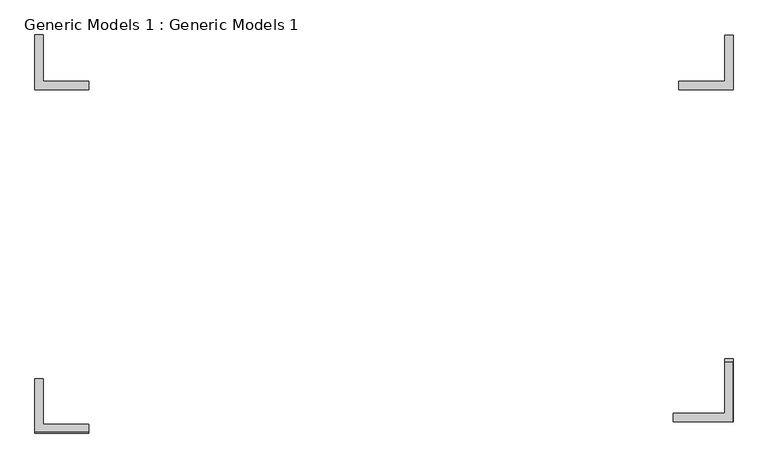
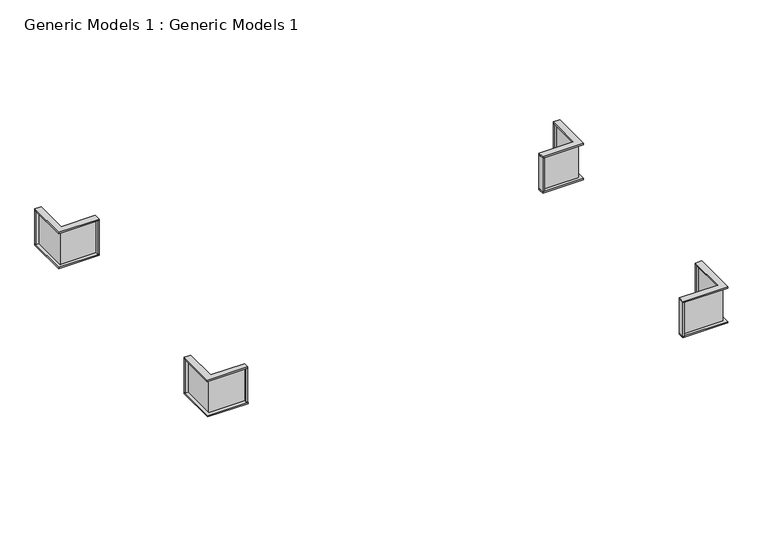
"""IFC4 building model written with IfcOpenShell, lengths in millimetres: proxy geometry, Generic Models 1 : Generic Models 1."""

from ifc_helpers import new_model, si_unit, frame, origin, place, context, project, spatial, polyline, outline, extrude, source, transform, mapped, element, save


def generic_models_1_generic_models_1_b24af07e(model_context):
    return source(origin(), model_context, "Body", "SweptSolid", [
        extrude(outline(polyline([(-6988.9378503, -5640.2673024), (-6988.9378503, -4368.6481466), (-6963.5378503, -4368.6481466), (-6963.5378503, -5614.8673024), (-5709.5498785, -5614.8673024), (-5709.5498785, -5640.2673024), (-6988.9378503, -5640.2673024)])), frame((0.0, 0.0, 4114.8), z_axis=(0.0, 0.0, 1.0), x_axis=(1.0, 0.0, 0.0)), (0.0, 0.0, 1.0), 1320.8),
        extrude(outline(polyline([(-6988.9378503, 3565.6135417), (-6988.9378503, 4868.3012615), (-6963.5378503, 4868.3012615), (-6963.5378503, 3591.0135417), (-5711.2501867, 3591.0135417), (-5711.2501867, 3565.6135417), (-6988.9378503, 3565.6135417)])), frame((0.0, 0.0, 4114.8), z_axis=(0.0, 0.0, 1.0), x_axis=(1.0, 0.0, 0.0)), (0.0, 0.0, 1.0), 1320.8),
        extrude(outline(polyline([(-7103.2378503, 4919.1012615), (-6874.6378503, 4919.1012615), (-6874.6378503, 4868.3012615), (-7103.2378503, 4868.3012615), (-7103.2378503, 4919.1012615)])), frame((0.0, 0.0, 4165.6), z_axis=(0.0, 0.0, 1.0), x_axis=(1.0, 0.0, 0.0)), (0.0, 0.0, 1.0), 1270.0),
        extrude(outline(polyline([(-5660.4501867, 3679.9135417), (-5660.4501867, 3451.3135417), (-5711.2501867, 3451.3135417), (-5711.2501867, 3679.9135417), (-5660.4501867, 3679.9135417)])), frame((0.0, 0.0, 4165.6), z_axis=(0.0, 0.0, 1.0), x_axis=(1.0, 0.0, 0.0)), (0.0, 0.0, 1.0), 1270.0),
        extrude(outline(polyline([(-7103.2378503, 3451.3135417), (-7103.2378503, 4919.1012615), (-6874.6378503, 4919.1012615), (-6874.6378503, 3679.9135417), (-5660.4501867, 3679.9135417), (-5660.4501867, 3451.3135417), (-7103.2378503, 3451.3135417)])), frame((0.0, 0.0, 5435.6), z_axis=(0.0, 0.0, 1.0), x_axis=(1.0, 0.0, 0.0)), (0.0, 0.0, 1.0), 50.8),
        extrude(outline(polyline([(-6874.6378503, 3679.9135417), (-5660.4501867, 3679.9135417), (-5660.4501867, 3451.3135417), (-7103.2378503, 3451.3135417), (-7103.2378503, 4919.1012615), (-6874.6378503, 4919.1012615), (-6874.6378503, 3679.9135417)])), frame((0.0, 0.0, 4114.8), z_axis=(0.0, 0.0, 1.0), x_axis=(1.0, 0.0, 0.0)), (0.0, 0.0, 1.0), 50.8),
        extrude(outline(polyline([(-5658.7498785, -5540.2864583), (-5658.7498785, -5740.2481466), (-5709.5498785, -5740.2481466), (-5709.5498785, -5540.2864583), (-5658.7498785, -5540.2864583)])), frame((0.0, 0.0, 4165.6), z_axis=(0.0, 0.0, 1.0), x_axis=(1.0, 0.0, 0.0)), (0.0, 0.0, 1.0), 1270.0),
        extrude(outline(polyline([(-7103.2378503, -4317.8481466), (-6874.6378503, -4317.8481466), (-6874.6378503, -4368.6481466), (-7103.2378503, -4368.6481466), (-7103.2378503, -4317.8481466)])), frame((0.0, 0.0, 4165.6), z_axis=(0.0, 0.0, 1.0), x_axis=(1.0, 0.0, 0.0)), (0.0, 0.0, 1.0), 1270.0),
        extrude(outline(polyline([(-7103.2378503, -5740.2481466), (-7103.2378503, -4317.8481466), (-6874.6378503, -4317.8481466), (-6874.6378503, -5540.2864583), (-5658.7498785, -5540.2864583), (-5658.7498785, -5740.2481466), (-7103.2378503, -5740.2481466)])), frame((0.0, 0.0, 5435.6), z_axis=(0.0, 0.0, 1.0), x_axis=(1.0, 0.0, 0.0)), (0.0, 0.0, 1.0), 50.8),
        extrude(outline(polyline([(-6874.6378503, -5540.2864583), (-5658.7498785, -5540.2864583), (-5658.7498785, -5768.8864583), (-7103.2378503, -5768.8864583), (-7103.2378503, -4317.8481466), (-6874.6378503, -4317.8481466), (-6874.6378503, -5540.2864583)])), frame((0.0, 0.0, 4114.8), z_axis=(0.0, 0.0, 1.0), x_axis=(1.0, 0.0, 0.0)), (0.0, 0.0, 1.0), 50.8),
        extrude(outline(polyline([(11524.4194554, -5350.7988103), (10090.1059555, -5350.7988103), (10090.1059555, -5325.3988103), (11499.0194554, -5325.3988103), (11499.0194554, -3918.1175755), (11524.4194554, -3918.1175755), (11524.4194554, -5350.7988103)])), frame((0.0, 0.0, 914.4), z_axis=(0.0, 0.0, 1.0), x_axis=(1.0, 0.0, 0.0)), (0.0, 0.0, 1.0), 1320.8),
        extrude(outline(polyline([(11527.6621497, 3565.6135417), (10236.8756044, 3565.6135417), (10236.8756044, 3591.0135417), (11502.2621497, 3591.0135417), (11502.2621497, 4866.0520795), (11527.6621497, 4866.0520795), (11527.6621497, 3565.6135417)])), frame((0.0, 0.0, 914.4), z_axis=(0.0, 0.0, 1.0), x_axis=(1.0, 0.0, 0.0)), (0.0, 0.0, 1.0), 1320.8),
        extrude(outline(polyline([(11413.3621497, 4916.8520795), (11641.9621497, 4916.8520795), (11641.9621497, 4866.0520795), (11413.3621497, 4866.0520795), (11413.3621497, 4916.8520795)])), frame((0.0, 0.0, 965.2), z_axis=(0.0, 0.0, 1.0), x_axis=(1.0, 0.0, 0.0)), (0.0, 0.0, 1.0), 1270.0),
        extrude(outline(polyline([(10186.0756044, 3451.3135417), (10186.0756044, 3679.9135417), (10236.8756044, 3679.9135417), (10236.8756044, 3451.3135417), (10186.0756044, 3451.3135417)])), frame((0.0, 0.0, 965.2), z_axis=(0.0, 0.0, 1.0), x_axis=(1.0, 0.0, 0.0)), (0.0, 0.0, 1.0), 1270.0),
        extrude(outline(polyline([(11413.3621497, 3679.9135417), (11413.3621497, 4916.8520795), (11641.9621497, 4916.8520795), (11641.9621497, 3451.3135417), (10186.0756044, 3451.3135417), (10186.0756044, 3679.9135417), (11413.3621497, 3679.9135417)])), frame((0.0, 0.0, 2235.2), z_axis=(0.0, 0.0, 1.0), x_axis=(1.0, 0.0, 0.0)), (0.0, 0.0, 1.0), 50.8),
        extrude(outline(polyline([(11413.3621497, 3679.9135417), (11413.3621497, 4916.8520795), (11641.9621497, 4916.8520795), (11641.9621497, 3451.3135417), (10186.0756044, 3451.3135417), (10186.0756044, 3679.9135417), (11413.3621497, 3679.9135417)])), frame((0.0, 0.0, 914.4), z_axis=(0.0, 0.0, 1.0), x_axis=(1.0, 0.0, 0.0)), (0.0, 0.0, 1.0), 50.8),
        extrude(outline(polyline([(10039.3059555, -5466.1111623), (10039.3059555, -5235.4864583), (10090.1059555, -5235.4864583), (10090.1059555, -5466.1111623), (10039.3059555, -5466.1111623)])), frame((0.0, 0.0, 965.2), z_axis=(0.0, 0.0, 1.0), x_axis=(1.0, 0.0, 0.0)), (0.0, 0.0, 1.0), 1270.0),
        extrude(outline(polyline([(11413.3621497, -3867.3175755), (11635.476761, -3867.3175755), (11635.476761, -3918.1175755), (11413.3621497, -3918.1175755), (11413.3621497, -3867.3175755)])), frame((0.0, 0.0, 972.5122471), z_axis=(0.0, 0.0, 1.0), x_axis=(1.0, 0.0, 0.0)), (0.0, 0.0, 1.0), 1262.6877529),
        extrude(outline(polyline([(11413.3621497, -5235.4864583), (11413.3621497, -3867.3175755), (11635.476761, -3859.5611623), (11635.476761, -5466.1111623), (10041.626761, -5466.1111623), (10041.626761, -5235.4864583), (11413.3621497, -5235.4864583)])), frame((0.0, 0.0, 2235.2), z_axis=(0.0, 0.0, 1.0), x_axis=(1.0, 0.0, 0.0)), (0.0, 0.0, 1.0), 50.8),
        extrude(outline(polyline([(11413.3621497, -5235.4864583), (11413.3621497, -3776.8981923), (11641.9621497, -3776.8981923), (11641.9621497, -5464.0864583), (10039.3059555, -5464.0864583), (10039.3059555, -5235.4864583), (11413.3621497, -5235.4864583)])), frame((0.0, 0.0, 914.4), z_axis=(0.0, 0.0, 1.0), x_axis=(1.0, 0.0, 0.0)), (0.0, 0.0, 1.0), 50.8),
    ])


if __name__ == "__main__":
    model = new_model("IFC4")
    model_context = context("Model", 3, world=origin())
    ifc_project = project(units=[si_unit("LENGTHUNIT", "METRE", prefix="MILLI")], contexts=[model_context])
    site = spatial("IfcSite", under=ifc_project)
    building = spatial("IfcBuilding", under=site)
    placement = place(None, origin())
    generic_models_1_generic_models_1_shape = generic_models_1_generic_models_1_b24af07e(model_context)
    element("IfcBuildingElementProxy", 1, Name="Generic Models 1 : Generic Models 1", ObjectType="Generic Models 1 : Generic Models 1", at=placement, inside=building, context=model_context, shape_type="MappedRepresentation", body=[
        mapped(generic_models_1_generic_models_1_shape, transform((0.0, 0.0, 0.0), x_axis=(1.0, 0.0, 0.0), y_axis=(0.0, 1.0, 0.0), z_axis=(0.0, 0.0, 1.0))),
    ])
    save(model, "model.ifc")

# Revit data of these elements
# Element 1 (IfcBuildingElementProxy, "Generic Models 1 : Generic Models 1")
#   Materials on its faces: "Door - Panel", "Glass - Clear, Grey"
# Materials
#   "Door - Panel": class "Wood", colour RGB 210 159 95, transparency 0, Cost = 0
#   "Glass - Clear, Grey": class "Glass", colour RGB 252 255 255, transparency 0.64
